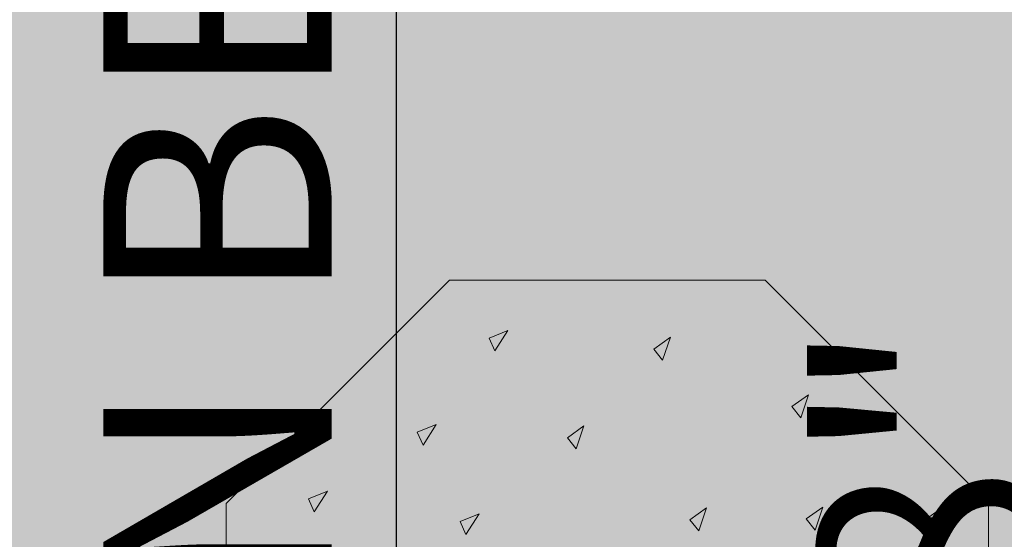
# Model space of a CAD drawing. Units: inches. Extents: x 459864 to 460310, y 324185 to 324787.
# Tile 54 of 112: x 460127 to 460153, y 324225 to 324239. Entities that reach past the tile are written whole.
import ezdxf

# ---------------------------------------------------------------- set-up
doc = ezdxf.new("R2010")
doc.units = ezdxf.units.IN
for name, color, linetype, lineweight in [('A-ANNO-DIMS', 2, 'Continuous', 18), ('L-HRDS', 9, 'Continuous', 18), ('L-SITE-PATT', 252, 'Continuous', 13)]:
    doc.layers.add(name, color=color, linetype=linetype, lineweight=lineweight)
doc.styles.get("Standard").update_dxf_attribs({"font": 'arial.ttf'})
doc.dimstyles.new('ISO-25', dxfattribs={"dimtxt": 6, "dimasz": 2.5, "dimexe": 1.25, "dimexo": 0.625, "dimtad": 1, "dimdec": 1, "dimlunit": 3, "dimtxsty": 'Standard', "dimcen": 2.5, "dimadec": 0, "dimazin": 0, "dimtfac": 1, "dimtdec": 1, "dimtmove": 0, "dimatfit": 3, "dimfxl": 1, "dimarcsym": 0})

# ---------------------------------------------------------------- blocks, each defined once
blk = doc.blocks.new('Stepping Stone - hexagonal')
for p, q in [((-5.099, 10.067), (-10.964, 4.202)), ((3.195, 10.067), (-5.099, 10.067)), ((9.06, 4.202), (3.195, 10.067)), ((-3.564, 8.743), (-4.061, 8.544)), ((-4.061, 8.544), (-3.906, 8.205)), ((-3.906, 8.205), (-3.564, 8.743)), ((0.704, 8.565), (0.267, 8.256)), ((0.497, 7.962), (0.704, 8.565)), ((0.267, 8.256), (0.497, 7.962)), ((4.333, 7.053), (3.895, 6.744)), ((4.125, 6.45), (4.333, 7.053)), ((3.895, 6.744), (4.125, 6.45)), ((-5.451, 6.27), (-5.948, 6.072)), ((-5.793, 5.732), (-5.451, 6.27)), ((-1.567, 6.236), (-2.004, 5.927)), ((-1.775, 5.633), (-1.567, 6.236)), ((-5.948, 6.072), (-5.793, 5.732)), ((-2.004, 5.927), (-1.775, 5.633)), ((-8.308, 4.52), (-8.806, 4.321)), ((-8.651, 3.982), (-8.308, 4.52)), ((-10.964, 4.202), (-10.964, -4.092)), ((-8.806, 4.321), (-8.651, 3.982)), ((9.06, -4.092), (9.06, 4.202)), ((-4.324, 3.923), (-4.821, 3.724)), ((-4.667, 3.385), (-4.324, 3.923)), ((1.654, 4.081), (1.217, 3.772)), ((1.447, 3.478), (1.654, 4.081)), ((4.709, 4.105), (4.272, 3.796)), ((4.502, 3.502), (4.709, 4.105)), ((7.74, 4.013), (7.303, 3.705)), ((7.532, 3.411), (7.74, 4.013)), ((-4.821, 3.724), (-4.667, 3.385)), ((1.217, 3.772), (1.447, 3.478)), ((4.272, 3.796), (4.502, 3.502)), ((7.303, 3.705), (7.532, 3.411))]:
    blk.add_line(p, q)
blk = doc.blocks.new('*D28')
at = {"layer": 'A-ANNO-DIMS', "color": 0, "lineweight": -2, "transparency": 16777216}
for p, q in [((460148.65, 324370.7), (460136.025, 324370.7)), ((460137.275, 324368.2), (460137.275, 324293.2)), ((460148.65, 324290.7), (460136.025, 324290.7)), ((460137.275, 324290.7), (460137.275, 324198.69))]:
    blk.add_line(p, q, dxfattribs=at)
at = {"layer": 'A-ANNO-DIMS', "color": 0, "transparency": 16777216}
for points in [[(460136.858, 324368.2), (460137.692, 324368.2), (460137.275, 324370.7)], [(460136.858, 324293.2), (460137.692, 324293.2), (460137.275, 324290.7)]]:
    blk.add_solid(points, dxfattribs=at)
at = {"layer": 'Defpoints', "color": 0, "transparency": 16777216}
for p in [(460149.275, 324370.7), (460137.275, 324290.7), (460149.275, 324290.7)]:
    blk.add_point(p, dxfattribs=at)
at = {"layer": 'A-ANNO-DIMS', "color": 0, "transparency": 16777216, "insert": (460133.363, 324243.445), "char_height": 6, "attachment_point": 5, "rotation": 90}
blk.add_mtext('QUEEN BED 6\'-8" TYP.', dxfattribs=at)
blk = doc.blocks.new('*D35')
at = {"layer": 'A-ANNO-DIMS', "color": 0, "lineweight": -2, "transparency": 16777216}
for p, q in [((460153.463, 324231.712), (460157.092, 324231.712)), ((460155.842, 324214.188), (460155.842, 324229.212)), ((460153.463, 324211.688), (460157.092, 324211.688))]:
    blk.add_line(p, q, dxfattribs=at)
at = {"layer": 'A-ANNO-DIMS', "color": 0, "transparency": 16777216}
for points in [[(460155.425, 324229.212), (460156.258, 324229.212), (460155.842, 324231.712)], [(460155.425, 324214.188), (460156.258, 324214.188), (460155.842, 324211.688)]]:
    blk.add_solid(points, dxfattribs=at)
at = {"layer": 'Defpoints', "color": 0, "transparency": 16777216}
for p in [(460152.838, 324231.712), (460155.842, 324231.712), (460152.838, 324211.688)]:
    blk.add_point(p, dxfattribs=at)
at = {"layer": 'A-ANNO-DIMS', "color": 0, "transparency": 16777216, "insert": (460152.153, 324221.7), "char_height": 6, "attachment_point": 5, "rotation": 90}
blk.add_mtext('1\'-8"', dxfattribs=at)

msp = doc.modelspace()

# ---------------------------------------------------------------- hatches: boundary and pattern name
at = {"layer": 'L-SITE-PATT'}
h = msp.add_hatch(dxfattribs=at)
h.set_pattern_fill('DOTS', color=256)
h.paths.add_polyline_path([(460269.804, 324283.483), (460247.115, 324283.483), (460121.929, 324283.483), (460121.929, 324252.473), (460117.429, 324252.473), (460110.124, 324252.473), (460110.124, 324243.287), (460080.83, 324243.287), (460080.83, 324252.473), (460061.115, 324252.473), (460061.115, 324251.882), (460077.909, 324251.882), (460077.909, 324199.483), (460080.83, 324199.483), (460080.83, 324207.553), (460110.124, 324207.553), (460110.124, 324199.483), (460110.813, 324199.483), (460262.115, 324199.483), (460269.804, 324199.483)], flags=17)
edge = h.paths.add_edge_path(flags=0)
edge.add_ellipse((460222.59, 324263.813), major_axis=(-8.485, 8.485), ratio=1, start_angle=405, end_angle=495, ccw=False)
edge.add_line((460214.821, 324254.66), (460214.832, 324254.666))
edge.add_ellipse((460222.59, 324263.813), major_axis=(-8.485, 8.485), ratio=1, start_angle=405, end_angle=495, ccw=False)
edge.add_line((460210.759, 324261.781), (460210.768, 324261.787))
edge.add_ellipse((460222.59, 324263.813), major_axis=(-8.485, 8.485), ratio=1, start_angle=405, end_angle=495, ccw=False)
edge.add_ellipse((460222.59, 324263.813), major_axis=(-8.485, 8.485), ratio=1, start_angle=392.754, end_angle=405, ccw=False)
edge.add_ellipse((460222.59, 324263.813), major_axis=(-8.485, 8.485), ratio=1, start_angle=380.9347, end_angle=392.754, ccw=False)
edge.add_line((460211.337, 324267.985), (460211.34, 324267.985))
edge.add_ellipse((460222.59, 324263.813), major_axis=(-8.485, 8.485), ratio=1, start_angle=380.9347, end_angle=392.754, ccw=False)
edge.add_ellipse((460222.59, 324263.813), major_axis=(-8.485, 8.485), ratio=1, start_angle=347.9015, end_angle=380.9347, ccw=False)
edge.add_ellipse((460222.59, 324263.813), major_axis=(-8.485, 8.485), ratio=1, start_angle=327.0619, end_angle=347.9015, ccw=False)
edge.add_ellipse((460222.59, 324263.813), major_axis=(-8.485, 8.485), ratio=1, start_angle=278.3246, end_angle=327.0619, ccw=False)
edge.add_line((460225.158, 324275.536), (460225.158, 324275.535))
edge.add_ellipse((460222.59, 324263.813), major_axis=(-8.485, 8.485), ratio=1, start_angle=278.3246, end_angle=327.0619, ccw=False)
edge.add_ellipse((460222.59, 324263.813), major_axis=(-8.485, 8.485), ratio=1, start_angle=260.6436, end_angle=278.3246, ccw=False)
edge.add_ellipse((460222.59, 324263.813), major_axis=(-8.485, 8.485), ratio=1, start_angle=225, end_angle=260.6436, ccw=False)
edge.add_line((460234.509, 324265.243), (460234.501, 324265.239))
edge.add_ellipse((460222.59, 324263.813), major_axis=(-8.485, 8.485), ratio=1, start_angle=225, end_angle=260.6436, ccw=False)
edge.add_ellipse((460222.59, 324263.813), major_axis=(-8.485, 8.485), ratio=1, start_angle=495, end_angle=585, ccw=False)
edge.add_line((460234.437, 324261.861), (460234.424, 324261.858))
edge.add_ellipse((460222.59, 324263.813), major_axis=(-8.485, 8.485), ratio=1, start_angle=495, end_angle=585, ccw=False)
edge.add_line((460227.95, 324253.067), (460227.946, 324253.083))
edge.add_ellipse((460222.59, 324263.813), major_axis=(-8.485, 8.485), ratio=1, start_angle=495, end_angle=585, ccw=False)
edge.add_line((460226.223, 324252.369), (460226.211, 324252.38))
edge.add_ellipse((460222.59, 324263.813), major_axis=(-8.485, 8.485), ratio=1, start_angle=495, end_angle=585, ccw=False)
h.paths.add_polyline_path([(460219.651, 324254.347), (460218.461, 324253.545), (460218.275, 324254.789), (460219.642, 324256.542), (460219.625, 324260.848), (460216.11, 324257.333), (460214.35, 324256.978), (460215.416, 324259.356), (460212.524, 324258.496), (460213.137, 324259.93), (460218.507, 324263.813), (460222.59, 324263.813), (460222.59, 324267.807), (460218.176, 324272.212), (460219.026, 324274.639), (460222.59, 324272.811), (460222.59, 324275.423), (460223.057, 324274.825), (460222.675, 324273.492), (460225.912, 324267.135), (460219.625, 324260.848)], flags=0)
edge = h.paths.add_edge_path(flags=0)
edge.add_ellipse((460194.576, 324264.046), major_axis=(-8.485, 8.485), ratio=1, start_angle=495, end_angle=585, ccw=False)
edge.add_line((460199.936, 324253.3), (460199.932, 324253.316))
edge.add_ellipse((460194.576, 324264.046), major_axis=(-8.485, 8.485), ratio=1, start_angle=495, end_angle=585, ccw=False)
edge.add_line((460198.208, 324252.603), (460198.196, 324252.613))
edge.add_ellipse((460194.576, 324264.046), major_axis=(-8.485, 8.485), ratio=1, start_angle=495, end_angle=585, ccw=False)
edge.add_ellipse((460194.576, 324264.046), major_axis=(-8.485, 8.485), ratio=1, start_angle=405, end_angle=495, ccw=False)
edge.add_line((460186.806, 324254.893), (460186.817, 324254.899))
edge.add_ellipse((460194.576, 324264.046), major_axis=(-8.485, 8.485), ratio=1, start_angle=405, end_angle=495, ccw=False)
edge.add_line((460182.744, 324262.014), (460182.753, 324262.02))
edge.add_ellipse((460194.576, 324264.046), major_axis=(-8.485, 8.485), ratio=1, start_angle=405, end_angle=495, ccw=False)
edge.add_ellipse((460194.576, 324264.046), major_axis=(-8.485, 8.485), ratio=1, start_angle=392.754, end_angle=405, ccw=False)
edge.add_ellipse((460194.576, 324264.046), major_axis=(-8.485, 8.485), ratio=1, start_angle=380.9347, end_angle=392.754, ccw=False)
edge.add_line((460183.323, 324268.218), (460183.326, 324268.218))
edge.add_ellipse((460194.576, 324264.046), major_axis=(-8.485, 8.485), ratio=1, start_angle=380.9347, end_angle=392.754, ccw=False)
edge.add_ellipse((460194.576, 324264.046), major_axis=(-8.485, 8.485), ratio=1, start_angle=347.9015, end_angle=380.9347, ccw=False)
edge.add_ellipse((460194.576, 324264.046), major_axis=(-8.485, 8.485), ratio=1, start_angle=327.0619, end_angle=347.9015, ccw=False)
edge.add_ellipse((460194.576, 324264.046), major_axis=(-8.485, 8.485), ratio=1, start_angle=278.3246, end_angle=327.0619, ccw=False)
edge.add_line((460197.144, 324275.769), (460197.143, 324275.768))
edge.add_ellipse((460194.576, 324264.046), major_axis=(-8.485, 8.485), ratio=1, start_angle=278.3246, end_angle=327.0619, ccw=False)
edge.add_ellipse((460194.576, 324264.046), major_axis=(-8.485, 8.485), ratio=1, start_angle=260.6436, end_angle=278.3246, ccw=False)
edge.add_ellipse((460194.576, 324264.046), major_axis=(-8.485, 8.485), ratio=1, start_angle=225, end_angle=260.6436, ccw=False)
edge.add_line((460206.494, 324265.476), (460206.487, 324265.473))
edge.add_ellipse((460194.576, 324264.046), major_axis=(-8.485, 8.485), ratio=1, start_angle=225, end_angle=260.6436, ccw=False)
edge.add_ellipse((460194.576, 324264.046), major_axis=(-8.485, 8.485), ratio=1, start_angle=495, end_angle=585, ccw=False)
edge.add_line((460206.422, 324262.094), (460206.409, 324262.091))
h.paths.add_polyline_path([(460191.61, 324261.081), (460191.637, 324254.58), (460190.447, 324253.778), (460190.261, 324255.023), (460191.628, 324256.775), (460191.61, 324261.081), (460188.096, 324257.566), (460186.335, 324257.211), (460187.402, 324259.589), (460184.509, 324258.729), (460185.123, 324260.163), (460190.493, 324264.046), (460194.576, 324264.046), (460194.576, 324268.04), (460190.161, 324272.446), (460191.011, 324274.872), (460194.576, 324273.044), (460194.576, 324275.657), (460195.043, 324275.058), (460194.661, 324273.725), (460197.897, 324267.368)], flags=0)
edge = h.paths.add_edge_path(flags=0)
edge.add_ellipse((460252.912, 324263.578), major_axis=(-8.485, 8.485), ratio=1, start_angle=405, end_angle=495, ccw=False)
edge.add_line((460241.081, 324261.545), (460241.089, 324261.551))
edge.add_ellipse((460252.912, 324263.578), major_axis=(-8.485, 8.485), ratio=1, start_angle=405, end_angle=495, ccw=False)
edge.add_ellipse((460252.912, 324263.578), major_axis=(-8.485, 8.485), ratio=1, start_angle=392.754, end_angle=405, ccw=False)
edge.add_ellipse((460252.912, 324263.578), major_axis=(-8.485, 8.485), ratio=1, start_angle=380.9347, end_angle=392.754, ccw=False)
edge.add_line((460241.659, 324267.749), (460241.662, 324267.749))
edge.add_ellipse((460252.912, 324263.578), major_axis=(-8.485, 8.485), ratio=1, start_angle=380.9347, end_angle=392.754, ccw=False)
edge.add_ellipse((460252.912, 324263.578), major_axis=(-8.485, 8.485), ratio=1, start_angle=347.9015, end_angle=380.9347, ccw=False)
edge.add_ellipse((460252.912, 324263.578), major_axis=(-8.485, 8.485), ratio=1, start_angle=327.0619, end_angle=347.9015, ccw=False)
edge.add_ellipse((460252.912, 324263.578), major_axis=(-8.485, 8.485), ratio=1, start_angle=278.3246, end_angle=327.0619, ccw=False)
edge.add_line((460255.48, 324275.3), (460255.479, 324275.299))
edge.add_ellipse((460252.912, 324263.578), major_axis=(-8.485, 8.485), ratio=1, start_angle=278.3246, end_angle=327.0619, ccw=False)
edge.add_ellipse((460252.912, 324263.578), major_axis=(-8.485, 8.485), ratio=1, start_angle=260.6436, end_angle=278.3246, ccw=False)
edge.add_ellipse((460252.912, 324263.578), major_axis=(-8.485, 8.485), ratio=1, start_angle=225, end_angle=260.6436, ccw=False)
edge.add_line((460264.83, 324265.007), (460264.823, 324265.004))
edge.add_ellipse((460252.912, 324263.578), major_axis=(-8.485, 8.485), ratio=1, start_angle=225, end_angle=260.6436, ccw=False)
edge.add_ellipse((460252.912, 324263.578), major_axis=(-8.485, 8.485), ratio=1, start_angle=495, end_angle=585, ccw=False)
edge.add_line((460264.758, 324261.626), (460264.745, 324261.622))
edge.add_ellipse((460252.912, 324263.578), major_axis=(-8.485, 8.485), ratio=1, start_angle=495, end_angle=585, ccw=False)
edge.add_line((460258.272, 324252.832), (460258.268, 324252.848))
edge.add_ellipse((460252.912, 324263.578), major_axis=(-8.485, 8.485), ratio=1, start_angle=495, end_angle=585, ccw=False)
edge.add_line((460256.545, 324252.134), (460256.533, 324252.144))
edge.add_ellipse((460252.912, 324263.578), major_axis=(-8.485, 8.485), ratio=1, start_angle=495, end_angle=585, ccw=False)
edge.add_ellipse((460252.912, 324263.578), major_axis=(-8.485, 8.485), ratio=1, start_angle=405, end_angle=495, ccw=False)
edge.add_line((460245.143, 324254.424), (460245.153, 324254.43))
h.paths.add_polyline_path([(460244.672, 324256.742), (460245.738, 324259.12), (460242.846, 324258.26), (460243.459, 324259.694), (460248.829, 324263.578), (460252.912, 324263.578), (460252.912, 324267.571), (460248.497, 324271.977), (460249.348, 324274.403), (460252.912, 324272.576), (460252.912, 324275.188), (460253.379, 324274.589), (460252.997, 324273.257), (460256.233, 324266.899), (460249.946, 324260.612), (460249.973, 324254.111), (460248.783, 324253.309), (460248.597, 324254.554), (460249.964, 324256.306), (460249.946, 324260.612), (460246.432, 324257.097)], flags=0)
edge = h.paths.add_edge_path(flags=0)
edge.add_ellipse((460167.439, 324262.833), major_axis=(-8.485, 8.485), ratio=1, start_angle=495, end_angle=585, ccw=False)
edge.add_line((460172.799, 324252.087), (460172.795, 324252.103))
edge.add_ellipse((460167.439, 324262.833), major_axis=(-8.485, 8.485), ratio=1, start_angle=495, end_angle=585, ccw=False)
edge.add_line((460171.071, 324251.389), (460171.059, 324251.399))
edge.add_ellipse((460167.439, 324262.833), major_axis=(-8.485, 8.485), ratio=1, start_angle=495, end_angle=585, ccw=False)
edge.add_ellipse((460167.439, 324262.833), major_axis=(-8.485, 8.485), ratio=1, start_angle=405, end_angle=495, ccw=False)
edge.add_line((460159.669, 324253.679), (460159.68, 324253.685))
edge.add_ellipse((460167.439, 324262.833), major_axis=(-8.485, 8.485), ratio=1, start_angle=405, end_angle=495, ccw=False)
edge.add_line((460155.607, 324260.8), (460155.616, 324260.806))
edge.add_ellipse((460167.439, 324262.833), major_axis=(-8.485, 8.485), ratio=1, start_angle=405, end_angle=495, ccw=False)
edge.add_ellipse((460167.439, 324262.833), major_axis=(-8.485, 8.485), ratio=1, start_angle=392.754, end_angle=405, ccw=False)
edge.add_ellipse((460167.439, 324262.833), major_axis=(-8.485, 8.485), ratio=1, start_angle=380.9347, end_angle=392.754, ccw=False)
edge.add_line((460156.185, 324267.005), (460156.189, 324267.005))
edge.add_ellipse((460167.439, 324262.833), major_axis=(-8.485, 8.485), ratio=1, start_angle=380.9347, end_angle=392.754, ccw=False)
edge.add_ellipse((460167.439, 324262.833), major_axis=(-8.485, 8.485), ratio=1, start_angle=347.9015, end_angle=380.9347, ccw=False)
edge.add_ellipse((460167.439, 324262.833), major_axis=(-8.485, 8.485), ratio=1, start_angle=327.0619, end_angle=347.9015, ccw=False)
edge.add_ellipse((460167.439, 324262.833), major_axis=(-8.485, 8.485), ratio=1, start_angle=278.3246, end_angle=327.0619, ccw=False)
edge.add_line((460170.007, 324274.556), (460170.006, 324274.554))
edge.add_ellipse((460167.439, 324262.833), major_axis=(-8.485, 8.485), ratio=1, start_angle=278.3246, end_angle=327.0619, ccw=False)
edge.add_ellipse((460167.439, 324262.833), major_axis=(-8.485, 8.485), ratio=1, start_angle=260.6436, end_angle=278.3246, ccw=False)
edge.add_ellipse((460167.439, 324262.833), major_axis=(-8.485, 8.485), ratio=1, start_angle=225, end_angle=260.6436, ccw=False)
edge.add_line((460179.357, 324264.262), (460179.35, 324264.259))
edge.add_ellipse((460167.439, 324262.833), major_axis=(-8.485, 8.485), ratio=1, start_angle=225, end_angle=260.6436, ccw=False)
edge.add_ellipse((460167.439, 324262.833), major_axis=(-8.485, 8.485), ratio=1, start_angle=495, end_angle=585, ccw=False)
edge.add_line((460179.285, 324260.881), (460179.272, 324260.877))
h.paths.add_polyline_path([(460164.473, 324259.867), (460164.5, 324253.366), (460163.31, 324252.565), (460163.124, 324253.809), (460164.491, 324255.561), (460164.473, 324259.867), (460160.958, 324256.353), (460159.198, 324255.998), (460160.265, 324258.375), (460157.372, 324257.515), (460157.986, 324258.949), (460163.356, 324262.833), (460167.439, 324262.833), (460167.439, 324266.826), (460163.024, 324271.232), (460163.874, 324273.659), (460167.439, 324271.831), (460167.439, 324274.443), (460167.905, 324273.844), (460167.524, 324272.512), (460170.76, 324266.154)], flags=0)
edge = h.paths.add_edge_path(flags=0)
edge.add_ellipse((460140.758, 324262.37), major_axis=(-8.485, 8.485), ratio=1, start_angle=495, end_angle=585, ccw=False)
edge.add_line((460146.118, 324251.624), (460146.114, 324251.639))
edge.add_ellipse((460140.758, 324262.37), major_axis=(-8.485, 8.485), ratio=1, start_angle=495, end_angle=585, ccw=False)
edge.add_line((460144.391, 324250.926), (460144.379, 324250.936))
edge.add_ellipse((460140.758, 324262.37), major_axis=(-8.485, 8.485), ratio=1, start_angle=495, end_angle=585, ccw=False)
edge.add_ellipse((460140.758, 324262.37), major_axis=(-8.485, 8.485), ratio=1, start_angle=405, end_angle=495, ccw=False)
edge.add_line((460132.989, 324253.216), (460132.999, 324253.222))
edge.add_ellipse((460140.758, 324262.37), major_axis=(-8.485, 8.485), ratio=1, start_angle=405, end_angle=495, ccw=False)
edge.add_line((460128.927, 324260.337), (460128.935, 324260.343))
edge.add_ellipse((460140.758, 324262.37), major_axis=(-8.485, 8.485), ratio=1, start_angle=405, end_angle=495, ccw=False)
edge.add_ellipse((460140.758, 324262.37), major_axis=(-8.485, 8.485), ratio=1, start_angle=392.754, end_angle=405, ccw=False)
edge.add_ellipse((460140.758, 324262.37), major_axis=(-8.485, 8.485), ratio=1, start_angle=380.9347, end_angle=392.754, ccw=False)
edge.add_line((460129.505, 324266.541), (460129.508, 324266.541))
edge.add_ellipse((460140.758, 324262.37), major_axis=(-8.485, 8.485), ratio=1, start_angle=380.9347, end_angle=392.754, ccw=False)
edge.add_ellipse((460140.758, 324262.37), major_axis=(-8.485, 8.485), ratio=1, start_angle=347.9015, end_angle=380.9347, ccw=False)
edge.add_ellipse((460140.758, 324262.37), major_axis=(-8.485, 8.485), ratio=1, start_angle=327.0619, end_angle=347.9015, ccw=False)
edge.add_ellipse((460140.758, 324262.37), major_axis=(-8.485, 8.485), ratio=1, start_angle=278.3246, end_angle=327.0619, ccw=False)
edge.add_line((460143.326, 324274.092), (460143.325, 324274.091))
edge.add_ellipse((460140.758, 324262.37), major_axis=(-8.485, 8.485), ratio=1, start_angle=278.3246, end_angle=327.0619, ccw=False)
edge.add_ellipse((460140.758, 324262.37), major_axis=(-8.485, 8.485), ratio=1, start_angle=260.6436, end_angle=278.3246, ccw=False)
edge.add_ellipse((460140.758, 324262.37), major_axis=(-8.485, 8.485), ratio=1, start_angle=225, end_angle=260.6436, ccw=False)
edge.add_line((460152.677, 324263.799), (460152.669, 324263.796))
edge.add_ellipse((460140.758, 324262.37), major_axis=(-8.485, 8.485), ratio=1, start_angle=225, end_angle=260.6436, ccw=False)
edge.add_ellipse((460140.758, 324262.37), major_axis=(-8.485, 8.485), ratio=1, start_angle=495, end_angle=585, ccw=False)
edge.add_line((460152.604, 324260.418), (460152.592, 324260.414))
h.paths.add_polyline_path([(460137.792, 324259.404), (460137.819, 324252.903), (460136.629, 324252.101), (460136.443, 324253.346), (460137.81, 324255.098), (460137.792, 324259.404), (460134.278, 324255.889), (460132.518, 324255.534), (460133.584, 324257.912), (460130.692, 324257.052), (460131.305, 324258.486), (460136.675, 324262.37), (460140.758, 324262.37), (460140.758, 324266.363), (460136.343, 324270.769), (460137.194, 324273.195), (460140.758, 324271.367), (460140.758, 324273.98), (460141.225, 324273.381), (460140.843, 324272.049), (460144.079, 324265.691)], flags=0)
h.paths.add_polyline_path([(460110.124, 324227.414), (460080.83, 324227.414), (460080.83, 324235.484), (460110.124, 324235.484)], flags=16)
h.paths.add_polyline_path([(460110.124, 324220.797), (460110.124, 324212.727), (460080.83, 324212.727), (460080.83, 324220.797)], flags=16)
h.paths.add_polyline_path([(460269.804, 324283.483), (460247.115, 324283.483), (460121.929, 324283.483), (460121.929, 324252.473), (460117.429, 324252.473), (460110.124, 324252.473), (460110.124, 324243.287), (460080.83, 324243.287), (460080.83, 324252.473), (460061.115, 324252.473), (460061.115, 324251.882), (460077.909, 324251.882), (460077.909, 324199.483), (460080.83, 324199.483), (460080.83, 324207.553), (460110.124, 324207.553), (460110.124, 324199.483), (460262.115, 324199.483), (460269.804, 324199.483)], flags=17)
h.paths.add_polyline_path([(460219.651, 324254.347), (460218.461, 324253.545), (460218.275, 324254.789), (460219.642, 324256.542), (460219.625, 324260.848), (460216.11, 324257.333), (460214.35, 324256.978), (460215.416, 324259.356), (460212.524, 324258.496), (460213.137, 324259.93), (460218.507, 324263.813), (460222.59, 324263.813), (460220.18, 324266.223), (460215.461, 324265.308), (460211.835, 324266.137), (460216.247, 324267.985), (460218.418, 324267.985), (460222.59, 324263.813), (460222.59, 324267.807), (460218.176, 324272.212), (460219.026, 324274.639), (460222.59, 324272.811), (460222.59, 324275.423), (460223.057, 324274.825), (460222.675, 324273.492), (460225.912, 324267.135), (460222.59, 324263.813), (460231.383, 324263.813), (460228.485, 324262.488), (460224.425, 324261.978), (460228.68, 324257.724), (460228.966, 324254.791), (460227.142, 324256.537), (460227.542, 324254.819), (460227.333, 324253.614), (460222.59, 324259.985), (460222.59, 324255.497), (460221.377, 324256.541), (460220.576, 324261.799), (460219.625, 324260.848)], flags=0)
h.paths.add_polyline_path([(460199.127, 324256.77), (460199.528, 324255.052), (460199.319, 324253.848), (460194.576, 324260.218), (460194.576, 324255.73), (460193.363, 324256.774), (460192.561, 324262.032), (460191.61, 324261.081), (460191.637, 324254.58), (460190.447, 324253.778), (460190.261, 324255.023), (460191.628, 324256.775), (460191.61, 324261.081), (460188.096, 324257.566), (460186.335, 324257.211), (460187.402, 324259.589), (460184.509, 324258.729), (460185.123, 324260.163), (460190.493, 324264.046), (460194.576, 324264.046), (460192.166, 324266.456), (460187.446, 324265.541), (460183.82, 324266.37), (460188.232, 324268.218), (460190.404, 324268.218), (460194.576, 324264.046), (460194.576, 324268.04), (460190.161, 324272.446), (460191.011, 324274.872), (460194.576, 324273.044), (460194.576, 324275.657), (460195.043, 324275.058), (460194.661, 324273.725), (460197.897, 324267.368), (460194.576, 324264.046), (460203.368, 324264.046), (460200.47, 324262.721), (460196.411, 324262.212), (460200.665, 324257.957), (460200.951, 324255.024)], flags=0)
h.paths.add_polyline_path([(460244.672, 324256.742), (460245.738, 324259.12), (460242.846, 324258.26), (460243.459, 324259.694), (460248.829, 324263.578), (460252.912, 324263.578), (460250.502, 324265.987), (460245.783, 324265.072), (460242.156, 324265.901), (460246.568, 324267.749), (460248.74, 324267.749), (460252.912, 324263.578), (460252.912, 324267.571), (460248.497, 324271.977), (460249.348, 324274.403), (460252.912, 324272.576), (460252.912, 324275.188), (460253.379, 324274.589), (460252.997, 324273.257), (460256.233, 324266.899), (460252.912, 324263.578), (460261.705, 324263.578), (460258.806, 324262.252), (460254.747, 324261.743), (460259.002, 324257.488), (460259.288, 324254.555), (460257.463, 324256.301), (460257.864, 324254.583), (460257.655, 324253.379), (460252.912, 324259.749), (460252.912, 324255.261), (460251.699, 324256.305), (460250.897, 324261.563), (460249.946, 324260.612), (460249.973, 324254.111), (460248.783, 324253.309), (460248.597, 324254.554), (460249.964, 324256.306), (460249.946, 324260.612), (460246.432, 324257.097)], flags=0)
h.paths.add_polyline_path([(460173.528, 324256.743), (460173.814, 324253.811), (460171.99, 324255.556), (460172.39, 324253.838), (460172.182, 324252.634), (460167.439, 324259.004), (460167.439, 324254.516), (460166.226, 324255.56), (460165.424, 324260.818), (460164.473, 324259.867), (460164.5, 324253.366), (460163.31, 324252.565), (460163.124, 324253.809), (460164.491, 324255.561), (460164.473, 324259.867), (460160.958, 324256.353), (460159.198, 324255.998), (460160.265, 324258.375), (460157.372, 324257.515), (460157.986, 324258.949), (460163.356, 324262.833), (460167.439, 324262.833), (460165.029, 324265.243), (460160.309, 324264.327), (460156.683, 324265.156), (460161.095, 324267.005), (460163.267, 324267.005), (460167.439, 324262.833), (460167.439, 324266.826), (460163.024, 324271.232), (460163.874, 324273.659), (460167.439, 324271.831), (460167.439, 324274.443), (460167.905, 324273.844), (460167.524, 324272.512), (460170.76, 324266.154), (460167.439, 324262.833), (460176.231, 324262.833), (460173.333, 324261.507), (460169.274, 324260.998)], flags=0)
h.paths.add_polyline_path([(460146.848, 324256.28), (460147.134, 324253.347), (460145.31, 324255.093), (460145.71, 324253.375), (460145.501, 324252.171), (460140.758, 324258.541), (460140.758, 324254.053), (460139.545, 324255.097), (460138.744, 324260.355), (460137.792, 324259.404), (460137.819, 324252.903), (460136.629, 324252.101), (460136.443, 324253.346), (460137.81, 324255.098), (460137.792, 324259.404), (460134.278, 324255.889), (460132.518, 324255.534), (460133.584, 324257.912), (460130.692, 324257.052), (460131.305, 324258.486), (460136.675, 324262.37), (460140.758, 324262.37), (460138.348, 324264.779), (460133.629, 324263.864), (460130.002, 324264.693), (460134.414, 324266.541), (460136.586, 324266.541), (460140.758, 324262.37), (460140.758, 324266.363), (460136.343, 324270.769), (460137.194, 324273.195), (460140.758, 324271.367), (460140.758, 324273.98), (460141.225, 324273.381), (460140.843, 324272.049), (460144.079, 324265.691), (460140.758, 324262.37), (460149.551, 324262.37), (460146.653, 324261.044), (460142.593, 324260.535)], flags=0)
edge = h.paths.add_edge_path()
edge.add_line((460269.804, 324272.549), (460260.881, 324272.549))
edge.add_ellipse((460252.912, 324263.578), major_axis=(-8.485, 8.485), ratio=1, start_angle=260.6436, end_angle=273.3846, ccw=False)
edge.add_line((460262.283, 324271.092), (460262.261, 324271.091))
edge.add_ellipse((460252.912, 324263.578), major_axis=(-8.485, 8.485), ratio=1, start_angle=260.6436, end_angle=273.3846, ccw=False)
edge.add_ellipse((460252.912, 324263.578), major_axis=(-8.485, 8.485), ratio=1, start_angle=225, end_angle=260.6436, ccw=False)
edge.add_line((460263.609, 324269.063), (460263.572, 324269.058))
edge.add_ellipse((460252.912, 324263.578), major_axis=(-8.485, 8.485), ratio=1, start_angle=225, end_angle=260.6436, ccw=False)
edge.add_line((460264.615, 324266.306), (460264.585, 324266.305))
edge.add_ellipse((460252.912, 324263.578), major_axis=(-8.485, 8.485), ratio=1, start_angle=225, end_angle=260.6436, ccw=False)
edge.add_line((460264.83, 324265.007), (460264.823, 324265.004))
edge.add_ellipse((460252.912, 324263.578), major_axis=(-8.485, 8.485), ratio=1, start_angle=225, end_angle=260.6436, ccw=False)
edge.add_ellipse((460252.912, 324263.578), major_axis=(-8.485, 8.485), ratio=1, start_angle=495, end_angle=585, ccw=False)
edge.add_line((460264.758, 324261.626), (460264.745, 324261.622))
edge.add_ellipse((460252.912, 324263.578), major_axis=(-8.485, 8.485), ratio=1, start_angle=495, end_angle=585, ccw=False)
edge.add_line((460263.442, 324257.739), (460263.389, 324257.779))
edge.add_ellipse((460252.912, 324263.578), major_axis=(-8.485, 8.485), ratio=1, start_angle=495, end_angle=585, ccw=False)
edge.add_line((460258.128, 324252.744), (460258.102, 324252.779))
edge.add_ellipse((460252.912, 324263.578), major_axis=(-8.485, 8.485), ratio=1, start_angle=495, end_angle=585, ccw=False)
edge.add_line((460256.545, 324252.134), (460256.533, 324252.144))
edge.add_ellipse((460252.912, 324263.578), major_axis=(-8.485, 8.485), ratio=1, start_angle=495, end_angle=585, ccw=False)
edge.add_ellipse((460252.912, 324263.578), major_axis=(-8.485, 8.485), ratio=1, start_angle=405, end_angle=495, ccw=False)
edge.add_line((460250.594, 324251.78), (460250.605, 324251.82))
edge.add_ellipse((460252.912, 324263.578), major_axis=(-8.485, 8.485), ratio=1, start_angle=405, end_angle=495, ccw=False)
edge.add_line((460245.143, 324254.424), (460245.153, 324254.43))
edge.add_ellipse((460252.912, 324263.578), major_axis=(-8.485, 8.485), ratio=1, start_angle=405, end_angle=495, ccw=False)
edge.add_line((460243.525, 324256.059), (460243.56, 324256.091))
edge.add_ellipse((460252.912, 324263.578), major_axis=(-8.485, 8.485), ratio=1, start_angle=405, end_angle=495, ccw=False)
edge.add_line((460241.44, 324259.893), (460241.522, 324259.896))
edge.add_ellipse((460252.912, 324263.578), major_axis=(-8.485, 8.485), ratio=1, start_angle=405, end_angle=495, ccw=False)
edge.add_line((460241.081, 324261.545), (460241.089, 324261.551))
edge.add_ellipse((460252.912, 324263.578), major_axis=(-8.485, 8.485), ratio=1, start_angle=405, end_angle=495, ccw=False)
edge.add_ellipse((460252.912, 324263.578), major_axis=(-8.485, 8.485), ratio=1, start_angle=392.754, end_angle=405, ccw=False)
edge.add_line((460241.05, 324265.438), (460241.063, 324265.443))
edge.add_ellipse((460252.912, 324263.578), major_axis=(-8.485, 8.485), ratio=1, start_angle=392.754, end_angle=405, ccw=False)
edge.add_ellipse((460252.912, 324263.578), major_axis=(-8.485, 8.485), ratio=1, start_angle=380.9347, end_angle=392.754, ccw=False)
edge.add_line((460241.452, 324267.176), (460241.469, 324267.171))
edge.add_ellipse((460252.912, 324263.578), major_axis=(-8.485, 8.485), ratio=1, start_angle=380.9347, end_angle=392.754, ccw=False)
edge.add_line((460241.659, 324267.749), (460241.662, 324267.749))
edge.add_ellipse((460252.912, 324263.578), major_axis=(-8.485, 8.485), ratio=1, start_angle=380.9347, end_angle=392.754, ccw=False)
edge.add_ellipse((460252.912, 324263.578), major_axis=(-8.485, 8.485), ratio=1, start_angle=356.6154, end_angle=380.9347, ccw=False)
edge.add_line((460244.88, 324272.488), (460244.713, 324272.549))
edge.add_line((460244.713, 324272.549), (460230.817, 324272.549))
edge.add_ellipse((460222.59, 324263.813), major_axis=(-8.485, 8.485), ratio=1, start_angle=260.6436, end_angle=271.7178, ccw=False)
edge.add_ellipse((460222.59, 324263.813), major_axis=(-8.485, 8.485), ratio=1, start_angle=225, end_angle=260.6436, ccw=False)
edge.add_line((460233.287, 324269.299), (460233.25, 324269.294))
edge.add_ellipse((460222.59, 324263.813), major_axis=(-8.485, 8.485), ratio=1, start_angle=225, end_angle=260.6436, ccw=False)
edge.add_line((460234.294, 324266.541), (460234.264, 324266.541))
edge.add_ellipse((460222.59, 324263.813), major_axis=(-8.485, 8.485), ratio=1, start_angle=225, end_angle=260.6436, ccw=False)
edge.add_line((460234.509, 324265.243), (460234.501, 324265.239))
edge.add_ellipse((460222.59, 324263.813), major_axis=(-8.485, 8.485), ratio=1, start_angle=225, end_angle=260.6436, ccw=False)
edge.add_ellipse((460222.59, 324263.813), major_axis=(-8.485, 8.485), ratio=1, start_angle=495, end_angle=585, ccw=False)
edge.add_line((460234.437, 324261.861), (460234.424, 324261.858))
edge.add_ellipse((460222.59, 324263.813), major_axis=(-8.485, 8.485), ratio=1, start_angle=495, end_angle=585, ccw=False)
edge.add_line((460233.121, 324257.975), (460233.068, 324258.015))
edge.add_ellipse((460222.59, 324263.813), major_axis=(-8.485, 8.485), ratio=1, start_angle=495, end_angle=585, ccw=False)
edge.add_line((460227.806, 324252.979), (460227.78, 324253.014))
edge.add_ellipse((460222.59, 324263.813), major_axis=(-8.485, 8.485), ratio=1, start_angle=495, end_angle=585, ccw=False)
edge.add_line((460226.223, 324252.369), (460226.211, 324252.38))
edge.add_ellipse((460222.59, 324263.813), major_axis=(-8.485, 8.485), ratio=1, start_angle=495, end_angle=585, ccw=False)
edge.add_ellipse((460222.59, 324263.813), major_axis=(-8.485, 8.485), ratio=1, start_angle=405, end_angle=495, ccw=False)
edge.add_line((460220.272, 324252.016), (460220.283, 324252.055))
edge.add_ellipse((460222.59, 324263.813), major_axis=(-8.485, 8.485), ratio=1, start_angle=405, end_angle=495, ccw=False)
edge.add_line((460214.821, 324254.66), (460214.832, 324254.666))
edge.add_ellipse((460222.59, 324263.813), major_axis=(-8.485, 8.485), ratio=1, start_angle=405, end_angle=495, ccw=False)
edge.add_line((460213.203, 324256.295), (460213.239, 324256.327))
edge.add_ellipse((460222.59, 324263.813), major_axis=(-8.485, 8.485), ratio=1, start_angle=405, end_angle=495, ccw=False)
edge.add_line((460211.118, 324260.128), (460211.201, 324260.131))
edge.add_ellipse((460222.59, 324263.813), major_axis=(-8.485, 8.485), ratio=1, start_angle=405, end_angle=495, ccw=False)
edge.add_line((460210.759, 324261.781), (460210.768, 324261.787))
edge.add_ellipse((460222.59, 324263.813), major_axis=(-8.485, 8.485), ratio=1, start_angle=405, end_angle=495, ccw=False)
edge.add_ellipse((460222.59, 324263.813), major_axis=(-8.485, 8.485), ratio=1, start_angle=392.754, end_angle=405, ccw=False)
edge.add_line((460210.729, 324265.673), (460210.741, 324265.678))
edge.add_ellipse((460222.59, 324263.813), major_axis=(-8.485, 8.485), ratio=1, start_angle=392.754, end_angle=405, ccw=False)
edge.add_ellipse((460222.59, 324263.813), major_axis=(-8.485, 8.485), ratio=1, start_angle=380.9347, end_angle=392.754, ccw=False)
edge.add_line((460211.13, 324267.412), (460211.147, 324267.407))
edge.add_ellipse((460222.59, 324263.813), major_axis=(-8.485, 8.485), ratio=1, start_angle=380.9347, end_angle=392.754, ccw=False)
edge.add_line((460211.337, 324267.985), (460211.34, 324267.985))
edge.add_ellipse((460222.59, 324263.813), major_axis=(-8.485, 8.485), ratio=1, start_angle=380.9347, end_angle=392.754, ccw=False)
edge.add_ellipse((460222.59, 324263.813), major_axis=(-8.485, 8.485), ratio=1, start_angle=358.2822, end_angle=380.9347, ccw=False)
edge.add_line((460213.705, 324271.902), (460213.709, 324271.869))
edge.add_ellipse((460222.59, 324263.813), major_axis=(-8.485, 8.485), ratio=1, start_angle=358.2822, end_angle=380.9347, ccw=False)
edge.add_line((460214.363, 324272.549), (460203.078, 324272.549))
edge.add_line((460203.078, 324272.549), (460203.06, 324272.531))
edge.add_ellipse((460194.576, 324264.046), major_axis=(-8.485, 8.485), ratio=1, start_angle=260.6436, end_angle=270.1168, ccw=False)
edge.add_line((460203.957, 324271.561), (460203.921, 324271.56))
edge.add_ellipse((460194.576, 324264.046), major_axis=(-8.485, 8.485), ratio=1, start_angle=260.6436, end_angle=270.1168, ccw=False)
edge.add_ellipse((460194.576, 324264.046), major_axis=(-8.485, 8.485), ratio=1, start_angle=225, end_angle=260.6436, ccw=False)
edge.add_line((460205.272, 324269.532), (460205.235, 324269.527))
edge.add_ellipse((460194.576, 324264.046), major_axis=(-8.485, 8.485), ratio=1, start_angle=225, end_angle=260.6436, ccw=False)
edge.add_line((460206.279, 324266.774), (460206.249, 324266.774))
edge.add_ellipse((460194.576, 324264.046), major_axis=(-8.485, 8.485), ratio=1, start_angle=225, end_angle=260.6436, ccw=False)
edge.add_line((460206.494, 324265.476), (460206.487, 324265.473))
edge.add_ellipse((460194.576, 324264.046), major_axis=(-8.485, 8.485), ratio=1, start_angle=225, end_angle=260.6436, ccw=False)
edge.add_ellipse((460194.576, 324264.046), major_axis=(-8.485, 8.485), ratio=1, start_angle=495, end_angle=585, ccw=False)
edge.add_line((460206.422, 324262.094), (460206.409, 324262.091))
edge.add_ellipse((460194.576, 324264.046), major_axis=(-8.485, 8.485), ratio=1, start_angle=495, end_angle=585, ccw=False)
edge.add_line((460205.106, 324258.208), (460205.053, 324258.248))
edge.add_ellipse((460194.576, 324264.046), major_axis=(-8.485, 8.485), ratio=1, start_angle=495, end_angle=585, ccw=False)
edge.add_line((460199.792, 324253.212), (460199.766, 324253.248))
edge.add_ellipse((460194.576, 324264.046), major_axis=(-8.485, 8.485), ratio=1, start_angle=495, end_angle=585, ccw=False)
edge.add_line((460198.208, 324252.603), (460198.196, 324252.613))
edge.add_ellipse((460194.576, 324264.046), major_axis=(-8.485, 8.485), ratio=1, start_angle=495, end_angle=585, ccw=False)
edge.add_ellipse((460194.576, 324264.046), major_axis=(-8.485, 8.485), ratio=1, start_angle=405, end_angle=495, ccw=False)
edge.add_line((460192.258, 324252.249), (460192.268, 324252.289))
edge.add_ellipse((460194.576, 324264.046), major_axis=(-8.485, 8.485), ratio=1, start_angle=405, end_angle=495, ccw=False)
edge.add_line((460186.806, 324254.893), (460186.817, 324254.899))
edge.add_ellipse((460194.576, 324264.046), major_axis=(-8.485, 8.485), ratio=1, start_angle=405, end_angle=495, ccw=False)
edge.add_line((460185.188, 324256.528), (460185.224, 324256.56))
edge.add_ellipse((460194.576, 324264.046), major_axis=(-8.485, 8.485), ratio=1, start_angle=405, end_angle=495, ccw=False)
edge.add_line((460183.104, 324260.362), (460183.186, 324260.365))
edge.add_ellipse((460194.576, 324264.046), major_axis=(-8.485, 8.485), ratio=1, start_angle=405, end_angle=495, ccw=False)
edge.add_line((460182.744, 324262.014), (460182.753, 324262.02))
edge.add_ellipse((460194.576, 324264.046), major_axis=(-8.485, 8.485), ratio=1, start_angle=405, end_angle=495, ccw=False)
edge.add_ellipse((460194.576, 324264.046), major_axis=(-8.485, 8.485), ratio=1, start_angle=392.754, end_angle=405, ccw=False)
edge.add_line((460182.714, 324265.906), (460182.726, 324265.912))
edge.add_ellipse((460194.576, 324264.046), major_axis=(-8.485, 8.485), ratio=1, start_angle=392.754, end_angle=405, ccw=False)
edge.add_ellipse((460194.576, 324264.046), major_axis=(-8.485, 8.485), ratio=1, start_angle=380.9347, end_angle=392.754, ccw=False)
edge.add_line((460183.116, 324267.645), (460183.133, 324267.64))
edge.add_ellipse((460194.576, 324264.046), major_axis=(-8.485, 8.485), ratio=1, start_angle=380.9347, end_angle=392.754, ccw=False)
edge.add_line((460183.323, 324268.218), (460183.326, 324268.218))
edge.add_ellipse((460194.576, 324264.046), major_axis=(-8.485, 8.485), ratio=1, start_angle=380.9347, end_angle=392.754, ccw=False)
edge.add_ellipse((460194.576, 324264.046), major_axis=(-8.485, 8.485), ratio=1, start_angle=359.8832, end_angle=380.9347, ccw=False)
edge.add_line((460184.491, 324270.611), (460184.553, 324270.611))
edge.add_ellipse((460194.576, 324264.046), major_axis=(-8.485, 8.485), ratio=1, start_angle=359.8832, end_angle=380.9347, ccw=False)
edge.add_line((460185.346, 324271.76), (460185.379, 324271.728))
edge.add_ellipse((460194.576, 324264.046), major_axis=(-8.485, 8.485), ratio=1, start_angle=359.8832, end_angle=380.9347, ccw=False)
edge.add_line((460185.697, 324272.086), (460185.633, 324272.549))
edge.add_line((460185.633, 324272.549), (460174.683, 324272.549))
edge.add_line((460174.683, 324272.549), (460174.606, 324272.457))
edge.add_ellipse((460167.439, 324262.833), major_axis=(-8.485, 8.485), ratio=1, start_angle=260.6436, end_angle=278.3246, ccw=False)
edge.add_ellipse((460167.439, 324262.833), major_axis=(-8.485, 8.485), ratio=1, start_angle=225, end_angle=260.6436, ccw=False)
edge.add_line((460178.135, 324268.318), (460178.098, 324268.313))
edge.add_ellipse((460167.439, 324262.833), major_axis=(-8.485, 8.485), ratio=1, start_angle=225, end_angle=260.6436, ccw=False)
edge.add_line((460179.142, 324265.561), (460179.112, 324265.56))
edge.add_ellipse((460167.439, 324262.833), major_axis=(-8.485, 8.485), ratio=1, start_angle=225, end_angle=260.6436, ccw=False)
edge.add_line((460179.357, 324264.262), (460179.35, 324264.259))
edge.add_ellipse((460167.439, 324262.833), major_axis=(-8.485, 8.485), ratio=1, start_angle=225, end_angle=260.6436, ccw=False)
edge.add_ellipse((460167.439, 324262.833), major_axis=(-8.485, 8.485), ratio=1, start_angle=495, end_angle=585, ccw=False)
edge.add_line((460179.285, 324260.881), (460179.272, 324260.877))
edge.add_ellipse((460167.439, 324262.833), major_axis=(-8.485, 8.485), ratio=1, start_angle=495, end_angle=585, ccw=False)
edge.add_line((460177.969, 324256.994), (460177.916, 324257.034))
edge.add_ellipse((460167.439, 324262.833), major_axis=(-8.485, 8.485), ratio=1, start_angle=495, end_angle=585, ccw=False)
edge.add_line((460172.655, 324251.999), (460172.629, 324252.034))
edge.add_ellipse((460167.439, 324262.833), major_axis=(-8.485, 8.485), ratio=1, start_angle=495, end_angle=585, ccw=False)
edge.add_line((460171.071, 324251.389), (460171.059, 324251.399))
edge.add_ellipse((460167.439, 324262.833), major_axis=(-8.485, 8.485), ratio=1, start_angle=495, end_angle=585, ccw=False)
edge.add_ellipse((460167.439, 324262.833), major_axis=(-8.485, 8.485), ratio=1, start_angle=405, end_angle=495, ccw=False)
edge.add_line((460165.121, 324251.036), (460165.131, 324251.075))
edge.add_ellipse((460167.439, 324262.833), major_axis=(-8.485, 8.485), ratio=1, start_angle=405, end_angle=495, ccw=False)
edge.add_line((460159.669, 324253.679), (460159.68, 324253.685))
edge.add_ellipse((460167.439, 324262.833), major_axis=(-8.485, 8.485), ratio=1, start_angle=405, end_angle=495, ccw=False)
edge.add_line((460158.051, 324255.314), (460158.087, 324255.347))
edge.add_ellipse((460167.439, 324262.833), major_axis=(-8.485, 8.485), ratio=1, start_angle=405, end_angle=495, ccw=False)
edge.add_line((460155.967, 324259.148), (460156.049, 324259.151))
edge.add_ellipse((460167.439, 324262.833), major_axis=(-8.485, 8.485), ratio=1, start_angle=405, end_angle=495, ccw=False)
edge.add_line((460155.607, 324260.8), (460155.616, 324260.806))
edge.add_ellipse((460167.439, 324262.833), major_axis=(-8.485, 8.485), ratio=1, start_angle=405, end_angle=495, ccw=False)
edge.add_ellipse((460167.439, 324262.833), major_axis=(-8.485, 8.485), ratio=1, start_angle=392.754, end_angle=405, ccw=False)
edge.add_line((460155.577, 324264.693), (460155.589, 324264.698))
edge.add_ellipse((460167.439, 324262.833), major_axis=(-8.485, 8.485), ratio=1, start_angle=392.754, end_angle=405, ccw=False)
edge.add_ellipse((460167.439, 324262.833), major_axis=(-8.485, 8.485), ratio=1, start_angle=380.9347, end_angle=392.754, ccw=False)
edge.add_line((460155.979, 324266.432), (460155.996, 324266.426))
edge.add_ellipse((460167.439, 324262.833), major_axis=(-8.485, 8.485), ratio=1, start_angle=380.9347, end_angle=392.754, ccw=False)
edge.add_line((460156.185, 324267.005), (460156.189, 324267.005))
edge.add_ellipse((460167.439, 324262.833), major_axis=(-8.485, 8.485), ratio=1, start_angle=380.9347, end_angle=392.754, ccw=False)
edge.add_ellipse((460167.439, 324262.833), major_axis=(-8.485, 8.485), ratio=1, start_angle=350.9345, end_angle=380.9347, ccw=False)
edge.add_line((460157.363, 324269.397), (460157.414, 324269.397))
edge.add_ellipse((460167.439, 324262.833), major_axis=(-8.485, 8.485), ratio=1, start_angle=350.9345, end_angle=380.9347, ccw=False)
edge.add_line((460158.221, 324270.535), (460158.236, 324270.519))
edge.add_ellipse((460167.439, 324262.833), major_axis=(-8.485, 8.485), ratio=1, start_angle=350.9345, end_angle=380.9347, ccw=False)
edge.add_line((460159.379, 324271.753), (460159.419, 324271.738))
edge.add_ellipse((460167.439, 324262.833), major_axis=(-8.485, 8.485), ratio=1, start_angle=350.9345, end_angle=380.9347, ccw=False)
edge.add_line((460160.396, 324272.549), (460147.112, 324272.549))
edge.add_ellipse((460140.758, 324262.37), major_axis=(-8.485, 8.485), ratio=1, start_angle=278.3246, end_angle=283.0261, ccw=False)
edge.add_ellipse((460140.758, 324262.37), major_axis=(-8.485, 8.485), ratio=1, start_angle=260.6436, end_angle=278.3246, ccw=False)
edge.add_ellipse((460140.758, 324262.37), major_axis=(-8.485, 8.485), ratio=1, start_angle=225, end_angle=260.6436, ccw=False)
edge.add_line((460151.455, 324267.855), (460151.418, 324267.85))
edge.add_ellipse((460140.758, 324262.37), major_axis=(-8.485, 8.485), ratio=1, start_angle=225, end_angle=260.6436, ccw=False)
edge.add_line((460152.462, 324265.098), (460152.431, 324265.097))
edge.add_ellipse((460140.758, 324262.37), major_axis=(-8.485, 8.485), ratio=1, start_angle=225, end_angle=260.6436, ccw=False)
edge.add_line((460152.677, 324263.799), (460152.669, 324263.796))
edge.add_ellipse((460140.758, 324262.37), major_axis=(-8.485, 8.485), ratio=1, start_angle=225, end_angle=260.6436, ccw=False)
edge.add_ellipse((460140.758, 324262.37), major_axis=(-8.485, 8.485), ratio=1, start_angle=495, end_angle=585, ccw=False)
edge.add_line((460152.604, 324260.418), (460152.592, 324260.414))
edge.add_ellipse((460140.758, 324262.37), major_axis=(-8.485, 8.485), ratio=1, start_angle=495, end_angle=585, ccw=False)
edge.add_line((460151.288, 324256.531), (460151.235, 324256.571))
edge.add_ellipse((460140.758, 324262.37), major_axis=(-8.485, 8.485), ratio=1, start_angle=495, end_angle=585, ccw=False)
edge.add_line((460145.974, 324251.535), (460145.948, 324251.571))
edge.add_ellipse((460140.758, 324262.37), major_axis=(-8.485, 8.485), ratio=1, start_angle=495, end_angle=585, ccw=False)
edge.add_line((460144.391, 324250.926), (460144.379, 324250.936))
edge.add_ellipse((460140.758, 324262.37), major_axis=(-8.485, 8.485), ratio=1, start_angle=495, end_angle=585, ccw=False)
edge.add_ellipse((460140.758, 324262.37), major_axis=(-8.485, 8.485), ratio=1, start_angle=405, end_angle=495, ccw=False)
edge.add_line((460138.44, 324250.572), (460138.451, 324250.612))
edge.add_ellipse((460140.758, 324262.37), major_axis=(-8.485, 8.485), ratio=1, start_angle=405, end_angle=495, ccw=False)
edge.add_line((460132.989, 324253.216), (460132.999, 324253.222))
edge.add_ellipse((460140.758, 324262.37), major_axis=(-8.485, 8.485), ratio=1, start_angle=405, end_angle=495, ccw=False)
edge.add_line((460131.371, 324254.851), (460131.406, 324254.883))
edge.add_ellipse((460140.758, 324262.37), major_axis=(-8.485, 8.485), ratio=1, start_angle=405, end_angle=495, ccw=False)
edge.add_line((460129.286, 324258.685), (460129.369, 324258.688))
edge.add_ellipse((460140.758, 324262.37), major_axis=(-8.485, 8.485), ratio=1, start_angle=405, end_angle=495, ccw=False)
edge.add_line((460128.927, 324260.337), (460128.935, 324260.343))
edge.add_ellipse((460140.758, 324262.37), major_axis=(-8.485, 8.485), ratio=1, start_angle=405, end_angle=495, ccw=False)
edge.add_ellipse((460140.758, 324262.37), major_axis=(-8.485, 8.485), ratio=1, start_angle=392.754, end_angle=405, ccw=False)
edge.add_line((460128.896, 324264.23), (460128.909, 324264.235))
edge.add_ellipse((460140.758, 324262.37), major_axis=(-8.485, 8.485), ratio=1, start_angle=392.754, end_angle=405, ccw=False)
edge.add_ellipse((460140.758, 324262.37), major_axis=(-8.485, 8.485), ratio=1, start_angle=380.9347, end_angle=392.754, ccw=False)
edge.add_line((460129.298, 324265.968), (460129.315, 324265.963))
edge.add_ellipse((460140.758, 324262.37), major_axis=(-8.485, 8.485), ratio=1, start_angle=380.9347, end_angle=392.754, ccw=False)
edge.add_line((460129.505, 324266.541), (460129.508, 324266.541))
edge.add_ellipse((460140.758, 324262.37), major_axis=(-8.485, 8.485), ratio=1, start_angle=380.9347, end_angle=392.754, ccw=False)
edge.add_ellipse((460140.758, 324262.37), major_axis=(-8.485, 8.485), ratio=1, start_angle=347.9015, end_angle=380.9347, ccw=False)
edge.add_line((460130.697, 324268.934), (460130.727, 324268.934))
edge.add_ellipse((460140.758, 324262.37), major_axis=(-8.485, 8.485), ratio=1, start_angle=347.9015, end_angle=380.9347, ccw=False)
edge.add_line((460131.869, 324270.48), (460131.879, 324270.413))
edge.add_ellipse((460140.758, 324262.37), major_axis=(-8.485, 8.485), ratio=1, start_angle=347.9015, end_angle=380.9347, ccw=False)
edge.add_line((460132.734, 324271.277), (460132.705, 324271.287))
edge.add_ellipse((460140.758, 324262.37), major_axis=(-8.485, 8.485), ratio=1, start_angle=347.9015, end_angle=380.9347, ccw=False)
edge.add_line((460134.24, 324272.445), (460134.204, 324272.549))
edge.add_line((460134.204, 324272.549), (460121.929, 324272.549))
edge.add_line((460121.929, 324272.549), (460121.929, 324252.473))
edge.add_line((460121.929, 324252.473), (460117.429, 324252.473))
edge.add_line((460117.429, 324252.473), (460110.124, 324252.473))
edge.add_line((460110.124, 324252.473), (460110.124, 324243.287))
edge.add_line((460110.124, 324243.287), (460080.83, 324243.287))
edge.add_line((460080.83, 324243.287), (460080.83, 324252.473))
edge.add_line((460080.83, 324252.473), (460061.115, 324252.473))
edge.add_line((460061.115, 324252.473), (460061.115, 324251.882))
edge.add_line((460061.115, 324251.882), (460077.909, 324251.882))
edge.add_line((460077.909, 324251.882), (460077.909, 324199.483))
edge.add_line((460077.909, 324199.483), (460080.83, 324199.483))
edge.add_line((460080.83, 324199.483), (460080.83, 324207.553))
edge.add_line((460080.83, 324207.553), (460110.124, 324207.553))
edge.add_line((460110.124, 324207.553), (460110.124, 324199.483))
edge.add_line((460110.124, 324199.483), (460110.813, 324199.483))
edge.add_line((460110.813, 324199.483), (460262.115, 324199.483))
edge.add_line((460262.115, 324199.483), (460269.804, 324199.483))
edge.add_line((460269.804, 324199.483), (460269.804, 324272.549))

# ---------------------------------------------------------------- block references
at = {"layer": 'L-HRDS'}
msp.add_blockref('Stepping Stone - hexagonal', (460143.778, 324221.645), dxfattribs=at)

# ---------------------------------------------------------------- dimensions: what is measured, and where the dimension line sits
at = {"layer": 'A-ANNO-DIMS'}
dim = msp.add_linear_dim(base=(460137.275, 324290.7), p1=(460149.275, 324370.7), p2=(460149.275, 324290.7), angle=270, text='QUEEN BED <> TYP.', dimstyle='ISO-25', override={"dimdec": 1, "dimlfac": 1, "dimrnd": 0, "dimzin": 1, "dimdsep": 46, "dimlunit": 4, "dimfrac": 2}, dxfattribs=at)
dim.commit()
dim.dimension.update_dxf_attribs({"geometry": '*D28', "text_midpoint": (460133.363, 324243.445)})
dim = msp.add_linear_dim(base=(460155.842, 324231.712), p1=(460152.838, 324211.688), p2=(460152.838, 324231.712), angle=90, dimstyle='ISO-25', override={"dimdec": 1, "dimlfac": 1, "dimrnd": 0, "dimzin": 1, "dimdsep": 46, "dimlunit": 4, "dimfrac": 2}, dxfattribs=at)
dim.commit()
dim.dimension.update_dxf_attribs({"geometry": '*D35', "text_midpoint": (460152.153, 324221.7)})

doc.saveas('drawing.dxf')
